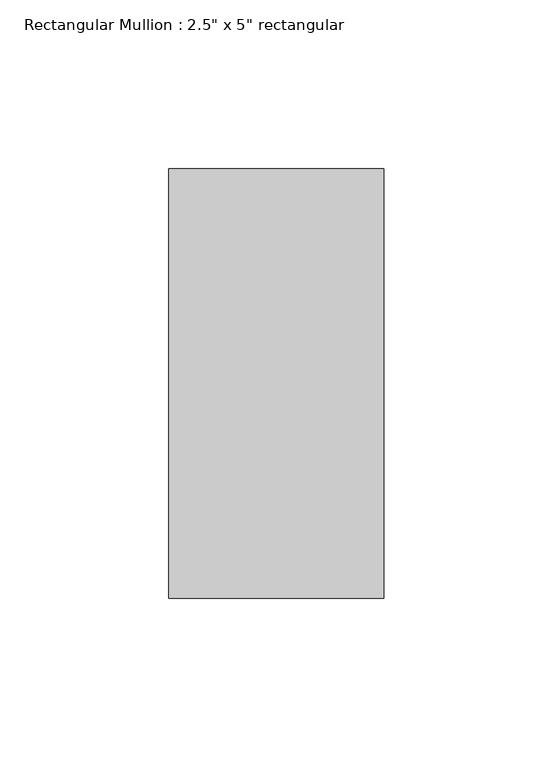
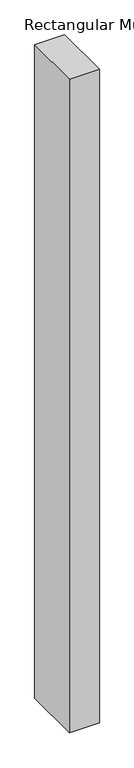
"""IFC4 building model written with IfcOpenShell, lengths in millimetres: member geometry."""

from ifc_helpers import new_model, si_unit, frame, origin, place, context, project, spatial, polyline, outline, extrude, source, transform, mapped, element, save


def member_e606cc0e(model_context):
    return source(origin(), model_context, "Body", "SweptSolid", [
        extrude(outline(polyline([(31.75, 63.5), (31.75, -63.5), (-31.75, -63.5), (-31.75, 63.5), (31.75, 63.5)])), frame((0.0, 0.0, -1462.4986146), z_axis=(0.0, 0.0, 1.0), x_axis=(1.0, 0.0, 0.0)), (0.0, 0.0, 1.0), 1462.4986146),
    ])


if __name__ == "__main__":
    model = new_model("IFC4")
    model_context = context("Model", 3, world=origin())
    ifc_project = project(units=[si_unit("LENGTHUNIT", "METRE", prefix="MILLI")], contexts=[model_context])
    site = spatial("IfcSite", under=ifc_project)
    building = spatial("IfcBuilding", under=site)
    placement = place(None, origin())
    member_shape = member_e606cc0e(model_context)
    element("IfcMember", 1, ObjectType="Rectangular Mullion : 2.5\" x 5\" rectangular", at=placement, inside=building, context=model_context, shape_type="MappedRepresentation", body=[
        mapped(member_shape, transform((0.0, 0.0, 0.0), x_axis=(1.0, 0.0, 0.0), y_axis=(0.0, 1.0, 0.0), z_axis=(0.0, 0.0, 1.0))),
    ])
    save(model, "model.ifc")

# Revit data of these elements
# Type "Rectangular Mullion : 2.5\" x 5\" rectangular"
#   built-in parameter 1007304 = 0.416667 (stored number, unit not read)
#   built-in parameter 1007301 = 0.104167 (stored number, unit not read)
#   built-in parameter 1007300 = 0.104167 (stored number, unit not read)
# Element 1 (IfcMember, "Rectangular Mullion : 2.5\" x 5\" rectangular")
#   Materials on its faces: "Aluminum"
# Materials
#   "Aluminum": class "Metal", colour RGB 247 247 247, transparency 0, Description = "Aluminum 6061", Cost = 0
